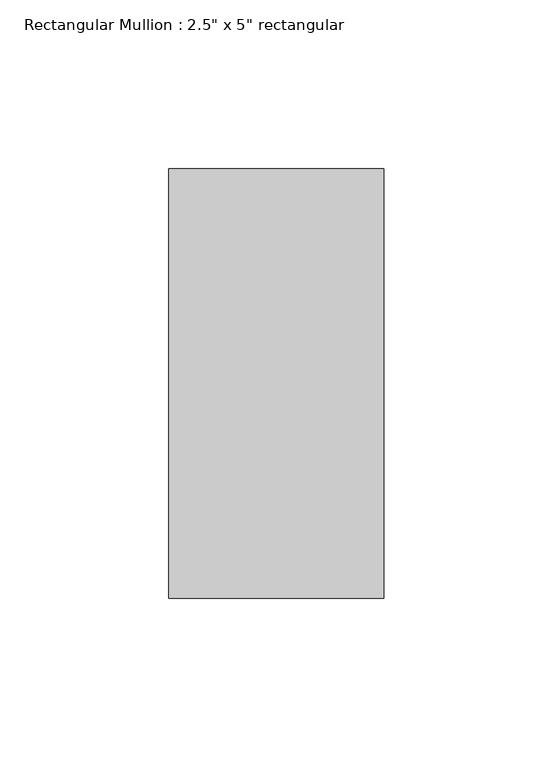
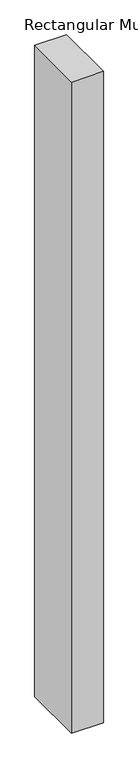
"""IFC4 building model written with IfcOpenShell, lengths in millimetres: member geometry."""

from ifc_helpers import new_model, si_unit, frame, origin, place, context, project, spatial, polyline, outline, extrude, source, transform, mapped, element, save


def member_824a4a8d(model_context):
    return source(origin(), model_context, "Body", "SweptSolid", [
        extrude(outline(polyline([(31.75, 63.5), (31.75, -63.5), (-31.75, -63.5), (-31.75, 63.5), (31.75, 63.5)])), frame((0.0, 0.0, -1371.6), z_axis=(0.0, 0.0, 1.0), x_axis=(1.0, 0.0, 0.0)), (0.0, 0.0, 1.0), 1371.6),
    ])


if __name__ == "__main__":
    model = new_model("IFC4")
    model_context = context("Model", 3, world=origin())
    ifc_project = project(units=[si_unit("LENGTHUNIT", "METRE", prefix="MILLI")], contexts=[model_context])
    site = spatial("IfcSite", under=ifc_project)
    building = spatial("IfcBuilding", under=site)
    placement = place(None, origin())
    member_shape = member_824a4a8d(model_context)
    element("IfcMember", 1, ObjectType="Rectangular Mullion : 2.5\" x 5\" rectangular", at=placement, inside=building, context=model_context, shape_type="MappedRepresentation", body=[
        mapped(member_shape, transform((0.0, 0.0, 0.0), x_axis=(1.0, 0.0, 0.0), y_axis=(0.0, 1.0, 0.0), z_axis=(0.0, 0.0, 1.0))),
    ])
    save(model, "model.ifc")

# Revit data of these elements
# Type "Rectangular Mullion : 2.5\" x 5\" rectangular"
#   built-in parameter 1007304 = 0.416667 (stored number, unit not read)
#   built-in parameter 1007301 = 0.104167 (stored number, unit not read)
#   built-in parameter 1007300 = 0.104167 (stored number, unit not read)
# Element 1 (IfcMember, "Rectangular Mullion : 2.5\" x 5\" rectangular")
#   Materials on its faces: "Aluminum"
# Materials
#   "Aluminum": class "Metal", colour RGB 247 247 247, transparency 0, Description = "Aluminum 6061", Cost = 0
